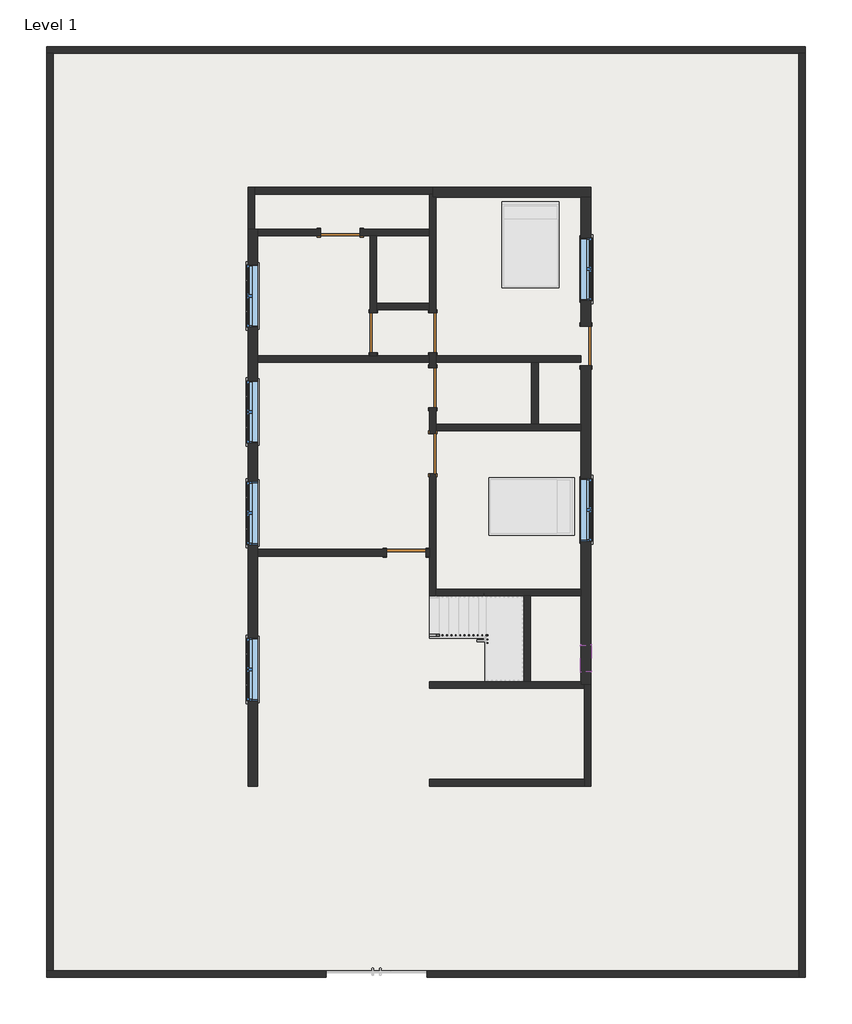
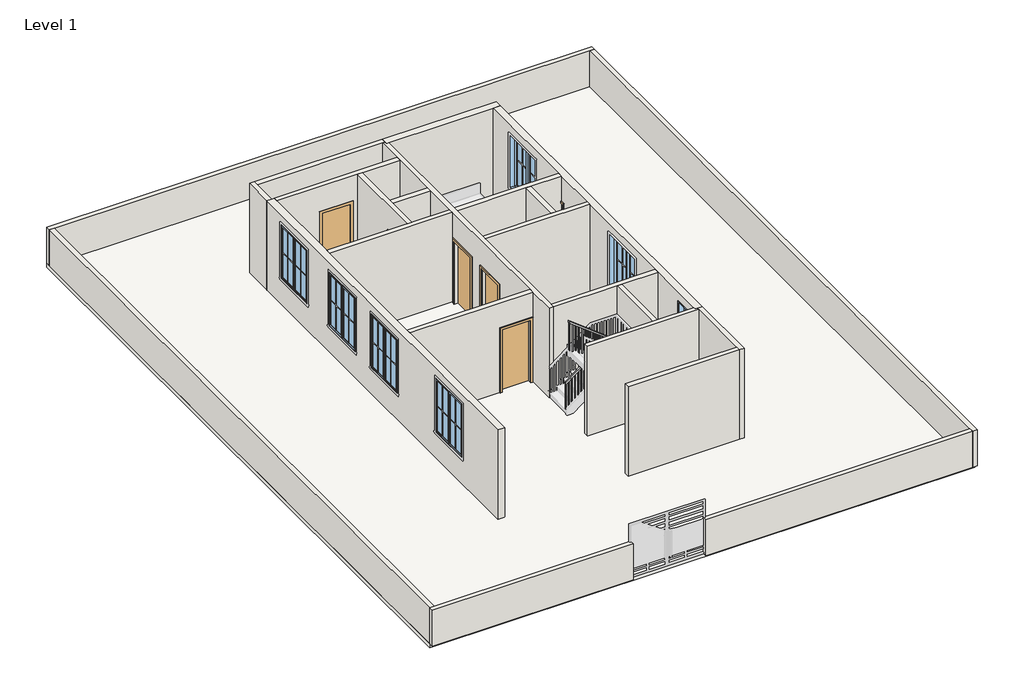
# One storey, part 1 of 2: 23 walls, 7 doors, 7 windows, 1 railing, 1 slab.
"""IFC4 building model written with IfcOpenShell, lengths in millimetres."""

from ifc_helpers import new_model, si_unit, frame, origin, origin_with_axes, place, context, project, spatial, polyline, outline, extrude, faceted_brep, transform, mapped, element, save
from components import door_686f89d2, door_16372e1c, door_0ca8825f, window_9ac97e1a, window_f2d8fef0

model = new_model("IFC4")

# Units and contexts
model_context = context("Model", 3, world=origin())
ifc_project = project(units=[si_unit("LENGTHUNIT", "METRE", prefix="MILLI")], contexts=[model_context])

# Site, building, storey
site = spatial("IfcSite", under=ifc_project)
building = spatial("IfcBuilding", under=site)
storey = spatial("IfcBuildingStorey", under=building, Name="Level 1", Elevation=0.0)

# Doors
placement = place(None, origin())
door_shape = door_686f89d2(model_context)
element("IfcDoor", 1, ObjectType="Single-Flush : 36\" x 84\"", at=placement, inside=storey, context=model_context, shape_type="MappedRepresentation", body=[
    mapped(door_shape, transform((-2318.0415352, 3143.9226491, 0.0), x_axis=(0.0, -1.0, 0.0), y_axis=(1.0, 0.0, 0.0), z_axis=(0.0, 0.0, 1.0))),
])
element("IfcDoor", 2, ObjectType="Single-Flush : 36\" x 84\"", at=placement, inside=storey, context=model_context, shape_type="MappedRepresentation", body=[
    mapped(door_shape, transform((-946.4415352, 3143.7222669, 0.0), x_axis=(0.0, 1.0, 0.0), y_axis=(-1.0, 0.0, 0.0), z_axis=(0.0, 0.0, 1.0))),
])
element("IfcDoor", 3, ObjectType="Single-Flush : 36\" x 84\"", at=placement, inside=storey, context=model_context, shape_type="MappedRepresentation", body=[
    mapped(door_shape, transform((-946.4415352, 1874.1230313, 0.0), x_axis=(0.0, 1.0, 0.0), y_axis=(-1.0, 0.0, 0.0), z_axis=(0.0, 0.0, 1.0))),
])
element("IfcDoor", 4, ObjectType="Single-Flush : 36\" x 84\"", at=placement, inside=storey, context=model_context, shape_type="MappedRepresentation", body=[
    mapped(door_shape, transform((-946.4415352, 350.1230313, 0.0), x_axis=(0.0, 1.0, 0.0), y_axis=(-1.0, 0.0, 0.0), z_axis=(0.0, 0.0, 1.0))),
])
element("IfcDoor", 5, ObjectType="Single-Flush : 36\" x 84\"", at=placement, inside=storey, context=model_context, shape_type="MappedRepresentation", body=[
    mapped(door_shape, transform((-3080.0415352, 5453.9645078, 0.0), x_axis=(1.0, 0.0, 0.0), y_axis=(0.0, 1.0, 0.0), z_axis=(0.0, 0.0, 1.0))),
])
door_2_shape = door_16372e1c(model_context)
element("IfcDoor", 6, ObjectType="Single-Flush : 36\" x 84\"", at=placement, inside=storey, context=model_context, shape_type="MappedRepresentation", body=[
    mapped(door_2_shape, transform((-1556.0415352, -1935.8769687, 0.0), x_axis=(1.0, 0.0, 0.0), y_axis=(0.0, 1.0, 0.0), z_axis=(0.0, 0.0, 1.0))),
])
door_3_shape = door_0ca8825f(model_context)
element("IfcDoor", 7, ObjectType="Single-Flush : 36\" x 84\"", at=placement, inside=storey, context=model_context, shape_type="MappedRepresentation", body=[
    mapped(door_3_shape, transform((2596.8584648, 2839.3230313, 0.0), x_axis=(0.0, -1.0, 0.0), y_axis=(1.0, 0.0, 0.0), z_axis=(0.0, 0.0, 1.0))),
])

# Railing
element("IfcRailing", 8, ObjectType="Handrail - Rectangular", at=placement, inside=storey, context=model_context, shape_type="SolidModel", body=[
    faceted_brep([(-1022.6415352, -3810.4539367, 1083.7333333), (-1022.6415352, -3810.4539367, 1019.5783974), (-1022.6415352, -3861.2539367, 1019.5783974), (-1022.6415352, -3861.2539367, 1083.7333333), (218.4221038, -3810.4539367, 2040.9605883), (269.2221038, -3810.4539367, 2015.9874824), (269.2221038, -3861.2539367, 2015.9874824), (218.4221038, -3861.2539367, 2040.9605883), (218.4221038, -3810.4539367, 2099.7333333), (269.2221038, -3810.4539367, 2048.9333333), (269.2221038, -3861.2539367, 2048.9333333), (218.4221038, -3861.2539367, 2099.7333333), (345.4221038, -3810.4539367, 2099.7333333), (345.4221038, -3810.4539367, 2048.9333333), (294.6221038, -3861.2539367, 2048.9333333), (294.6221038, -3861.2539367, 2099.7333333), (345.4221038, -3937.4539367, 2099.7333333), (345.4221038, -3937.4539367, 2048.9333333), (294.6221038, -3937.4539367, 2048.9333333), (294.6221038, -3937.4539367, 2099.7333333), (345.4221038, -3993.2769687, 2099.7333333), (294.6221038, -3993.2769687, 2099.7333333), (294.6221038, -4044.0769687, 2048.9333333), (345.4221038, -4044.0769687, 2048.9333333)], [[[0, 1, 2, 3]], [[1, 0, 4, 5]], [[2, 1, 5, 6]], [[3, 2, 6, 7]], [[0, 3, 7, 4]], [[5, 4, 8, 9]], [[6, 5, 9, 10]], [[7, 6, 10, 11]], [[4, 7, 11, 8]], [[9, 8, 12, 13]], [[10, 9, 13, 14]], [[11, 10, 14, 15]], [[8, 11, 15, 12]], [[13, 12, 16, 17]], [[14, 13, 17, 18]], [[15, 14, 18, 19]], [[12, 15, 19, 16]], [[20, 21, 22, 23]], [[17, 16, 20, 23]], [[18, 17, 23, 22]], [[19, 18, 22, 21]], [[16, 19, 21, 20]]]),
    faceted_brep([(345.4221038, -3993.2769687, 2099.7333333), (345.4221038, -4044.0769687, 2048.9333333), (294.6221038, -4044.0769687, 2048.9333333), (294.6221038, -3993.2769687, 2099.7333333), (345.4221038, -3993.2769687, 2229.8848366), (294.6221038, -3993.2769687, 2204.9117307), (294.6221038, -4044.0769687, 2204.9117307), (345.4221038, -4044.0769687, 2229.8848366)], [[[0, 1, 2, 3]], [[4, 5, 6, 7]], [[1, 0, 4, 7]], [[2, 1, 7, 6]], [[3, 2, 6, 5]], [[0, 3, 5, 4]]]),
    faceted_brep([(345.4221038, -4044.0769687, 2229.8848366), (294.6221038, -4044.0769687, 2204.9117307), (294.6221038, -3993.2769687, 2204.9117307), (345.4221038, -3993.2769687, 2229.8848366), (-1022.6415352, -4044.0769687, 3285.0666667), (-1022.6415352, -3993.2769687, 3285.0666667), (-1022.6415352, -3993.2769687, 3220.9117307), (-1022.6415352, -4044.0769687, 3220.9117307)], [[[0, 1, 2, 3]], [[4, 5, 6, 7]], [[1, 0, 4, 7]], [[2, 1, 7, 6]], [[3, 2, 6, 5]], [[0, 3, 5, 4]]]),
    extrude(outline(polyline([(3196.7018032, -991.2528962), (3211.3949894, -1010.3028962), (2201.3333333, -1010.3028962), (2201.3333333, -991.2528962), (3196.7018032, -991.2528962)])), frame((0.0, -4028.2019687, 0.0), z_axis=(0.0, 1.0, 0.0), x_axis=(0.0, 0.0, 1.0)), (0.0, 0.0, 1.0), 19.05),
    extrude(outline(polyline([(3118.3381431, -889.6528962), (3133.0313294, -908.7028962), (2201.3333333, -908.7028962), (2201.3333333, -889.6528962), (3118.3381431, -889.6528962)])), frame((0.0, -4028.2019687, 0.0), z_axis=(0.0, 1.0, 0.0), x_axis=(0.0, 0.0, 1.0)), (0.0, 0.0, 1.0), 19.05),
    extrude(outline(polyline([(3039.9744831, -788.0528962), (3054.6676694, -807.1028962), (2201.3333333, -807.1028962), (2201.3333333, -788.0528962), (3039.9744831, -788.0528962)])), frame((0.0, -4028.2019687, 0.0), z_axis=(0.0, 1.0, 0.0), x_axis=(0.0, 0.0, 1.0)), (0.0, 0.0, 1.0), 19.05),
    extrude(outline(polyline([(2961.6108231, -686.4528962), (2976.3040093, -705.5028962), (2032.0, -705.5028962), (2032.0, -686.4528962), (2961.6108231, -686.4528962)])), frame((0.0, -4028.2019687, 0.0), z_axis=(0.0, 1.0, 0.0), x_axis=(0.0, 0.0, 1.0)), (0.0, 0.0, 1.0), 19.05),
    extrude(outline(polyline([(2883.247163, -584.8528962), (2897.9403493, -603.9028962), (2032.0, -603.9028962), (2032.0, -584.8528962), (2883.247163, -584.8528962)])), frame((0.0, -4028.2019687, 0.0), z_axis=(0.0, 1.0, 0.0), x_axis=(0.0, 0.0, 1.0)), (0.0, 0.0, 1.0), 19.05),
    extrude(outline(polyline([(2804.883503, -483.2528962), (2819.5766892, -502.3028962), (1862.6666667, -502.3028962), (1862.6666667, -483.2528962), (2804.883503, -483.2528962)])), frame((0.0, -4028.2019687, 0.0), z_axis=(0.0, 1.0, 0.0), x_axis=(0.0, 0.0, 1.0)), (0.0, 0.0, 1.0), 19.05),
    extrude(outline(polyline([(2726.5198429, -381.6528962), (2741.2130292, -400.7028962), (1862.6666667, -400.7028962), (1862.6666667, -381.6528962), (2726.5198429, -381.6528962)])), frame((0.0, -4028.2019687, 0.0), z_axis=(0.0, 1.0, 0.0), x_axis=(0.0, 0.0, 1.0)), (0.0, 0.0, 1.0), 19.05),
    extrude(outline(polyline([(2648.1561829, -280.0528962), (2662.8493691, -299.1028962), (1693.3333333, -299.1028962), (1693.3333333, -280.0528962), (2648.1561829, -280.0528962)])), frame((0.0, -4028.2019687, 0.0), z_axis=(0.0, 1.0, 0.0), x_axis=(0.0, 0.0, 1.0)), (0.0, 0.0, 1.0), 19.05),
    extrude(outline(polyline([(2569.7925228, -178.4528962), (2584.4857091, -197.5028962), (1693.3333333, -197.5028962), (1693.3333333, -178.4528962), (2569.7925228, -178.4528962)])), frame((0.0, -4028.2019687, 0.0), z_axis=(0.0, 1.0, 0.0), x_axis=(0.0, 0.0, 1.0)), (0.0, 0.0, 1.0), 19.05),
    extrude(outline(polyline([(2491.4288628, -76.8528962), (2506.122049, -95.9028962), (1524.0, -95.9028962), (1524.0, -76.8528962), (2491.4288628, -76.8528962)])), frame((0.0, -4028.2019687, 0.0), z_axis=(0.0, 1.0, 0.0), x_axis=(0.0, 0.0, 1.0)), (0.0, 0.0, 1.0), 19.05),
    extrude(outline(polyline([(2413.0652027, 24.7471038), (2427.758389, 5.6971038), (1524.0, 5.6971038), (1524.0, 24.7471038), (2413.0652027, 24.7471038)])), frame((0.0, -4028.2019687, 0.0), z_axis=(0.0, 1.0, 0.0), x_axis=(0.0, 0.0, 1.0)), (0.0, 0.0, 1.0), 19.05),
    extrude(outline(polyline([(2334.7015427, 126.3471038), (2349.3947289, 107.2971038), (1524.0, 107.2971038), (1524.0, 126.3471038), (2334.7015427, 126.3471038)])), frame((0.0, -4028.2019687, 0.0), z_axis=(0.0, 1.0, 0.0), x_axis=(0.0, 0.0, 1.0)), (0.0, 0.0, 1.0), 19.05),
    extrude(outline(polyline([(2256.3378826, 227.9471038), (2271.0310689, 208.8971038), (1354.6666667, 208.8971038), (1354.6666667, 227.9471038), (2256.3378826, 227.9471038)])), frame((0.0, -4028.2019687, 0.0), z_axis=(0.0, 1.0, 0.0), x_axis=(0.0, 0.0, 1.0)), (0.0, 0.0, 1.0), 19.05),
    extrude(outline(polyline([(310.4971038, -3927.9289367), (329.5471038, -3927.9289367), (329.5471038, -3946.9789367), (310.4971038, -3946.9789367), (310.4971038, -3927.9289367)])), frame((0.0, 0.0, 1185.3333333), z_axis=(0.0, 0.0, 1.0), x_axis=(1.0, 0.0, 0.0)), (0.0, 0.0, 1.0), 863.6),
    extrude(outline(polyline([(288.6334648, -3845.3789367), (288.6334648, -3826.3289367), (307.6834648, -3826.3289367), (307.6834648, -3845.3789367), (288.6334648, -3845.3789367)])), frame((0.0, 0.0, 1185.3333333), z_axis=(0.0, 0.0, 1.0), x_axis=(1.0, 0.0, 0.0)), (0.0, 0.0, 1.0), 863.6),
    extrude(outline(polyline([(1967.2889111, 206.0834648), (1952.5957248, 187.0334648), (1016.0, 187.0334648), (1016.0, 206.0834648), (1967.2889111, 206.0834648)])), frame((0.0, -3845.3789367, 0.0), z_axis=(0.0, 1.0, 0.0), x_axis=(0.0, 0.0, 1.0)), (0.0, 0.0, 1.0), 19.05),
    extrude(outline(polyline([(1888.925251, 104.4834648), (1874.2320648, 85.4334648), (846.6666667, 85.4334648), (846.6666667, 104.4834648), (1888.925251, 104.4834648)])), frame((0.0, -3845.3789367, 0.0), z_axis=(0.0, 1.0, 0.0), x_axis=(0.0, 0.0, 1.0)), (0.0, 0.0, 1.0), 19.05),
    extrude(outline(polyline([(1810.561591, 2.8834648), (1795.8684047, -16.1665352), (846.6666667, -16.1665352), (846.6666667, 2.8834648), (1810.561591, 2.8834648)])), frame((0.0, -3845.3789367, 0.0), z_axis=(0.0, 1.0, 0.0), x_axis=(0.0, 0.0, 1.0)), (0.0, 0.0, 1.0), 19.05),
    extrude(outline(polyline([(1732.1979309, -98.7165352), (1717.5047447, -117.7665352), (846.6666667, -117.7665352), (846.6666667, -98.7165352), (1732.1979309, -98.7165352)])), frame((0.0, -3845.3789367, 0.0), z_axis=(0.0, 1.0, 0.0), x_axis=(0.0, 0.0, 1.0)), (0.0, 0.0, 1.0), 19.05),
    extrude(outline(polyline([(1653.8342709, -200.3165352), (1639.1410846, -219.3665352), (677.3333333, -219.3665352), (677.3333333, -200.3165352), (1653.8342709, -200.3165352)])), frame((0.0, -3845.3789367, 0.0), z_axis=(0.0, 1.0, 0.0), x_axis=(0.0, 0.0, 1.0)), (0.0, 0.0, 1.0), 19.05),
    extrude(outline(polyline([(1575.4706109, -301.9165352), (1560.7774246, -320.9665352), (677.3333333, -320.9665352), (677.3333333, -301.9165352), (1575.4706109, -301.9165352)])), frame((0.0, -3845.3789367, 0.0), z_axis=(0.0, 1.0, 0.0), x_axis=(0.0, 0.0, 1.0)), (0.0, 0.0, 1.0), 19.05),
    extrude(outline(polyline([(1497.1069508, -403.5165352), (1482.4137645, -422.5665352), (508.0, -422.5665352), (508.0, -403.5165352), (1497.1069508, -403.5165352)])), frame((0.0, -3845.3789367, 0.0), z_axis=(0.0, 1.0, 0.0), x_axis=(0.0, 0.0, 1.0)), (0.0, 0.0, 1.0), 19.05),
    extrude(outline(polyline([(1418.7432908, -505.1165352), (1404.0501045, -524.1665352), (508.0, -524.1665352), (508.0, -505.1165352), (1418.7432908, -505.1165352)])), frame((0.0, -3845.3789367, 0.0), z_axis=(0.0, 1.0, 0.0), x_axis=(0.0, 0.0, 1.0)), (0.0, 0.0, 1.0), 19.05),
    extrude(outline(polyline([(1340.3796307, -606.7165352), (1325.6864445, -625.7665352), (338.6666667, -625.7665352), (338.6666667, -606.7165352), (1340.3796307, -606.7165352)])), frame((0.0, -3845.3789367, 0.0), z_axis=(0.0, 1.0, 0.0), x_axis=(0.0, 0.0, 1.0)), (0.0, 0.0, 1.0), 19.05),
    extrude(outline(polyline([(1262.0159707, -708.3165352), (1247.3227844, -727.3665352), (338.6666667, -727.3665352), (338.6666667, -708.3165352), (1262.0159707, -708.3165352)])), frame((0.0, -3845.3789367, 0.0), z_axis=(0.0, 1.0, 0.0), x_axis=(0.0, 0.0, 1.0)), (0.0, 0.0, 1.0), 19.05),
    extrude(outline(polyline([(1183.6523106, -809.9165352), (1168.9591244, -828.9665352), (169.3333333, -828.9665352), (169.3333333, -809.9165352), (1183.6523106, -809.9165352)])), frame((0.0, -3845.3789367, 0.0), z_axis=(0.0, 1.0, 0.0), x_axis=(0.0, 0.0, 1.0)), (0.0, 0.0, 1.0), 19.05),
    extrude(outline(polyline([(1105.2886506, -911.5165352), (1090.5954643, -930.5665352), (169.3333333, -930.5665352), (169.3333333, -911.5165352), (1105.2886506, -911.5165352)])), frame((0.0, -3845.3789367, 0.0), z_axis=(0.0, 1.0, 0.0), x_axis=(0.0, 0.0, 1.0)), (0.0, 0.0, 1.0), 19.05),
    extrude(outline(polyline([(310.4971038, -4009.1519687), (329.5471038, -4009.1519687), (329.5471038, -4028.2019687), (310.4971038, -4028.2019687), (310.4971038, -4009.1519687)])), frame((0.0, 0.0, 1185.3333333), z_axis=(0.0, 0.0, 1.0), x_axis=(1.0, 0.0, 0.0)), (0.0, 0.0, 1.0), 863.6),
    extrude(outline(polyline([(310.4971038, -3845.3789367), (310.4971038, -3826.3289367), (329.5471038, -3826.3289367), (329.5471038, -3845.3789367), (310.4971038, -3845.3789367)])), frame((0.0, 0.0, 1185.3333333), z_axis=(0.0, 0.0, 1.0), x_axis=(1.0, 0.0, 0.0)), (0.0, 0.0, 1.0), 863.6),
    extrude(outline(polyline([(3206.2185445, -1003.5915352), (3220.9117307, -1022.6415352), (2201.3333333, -1022.6415352), (2201.3333333, -1003.5915352), (3206.2185445, -1003.5915352)])), frame((0.0, -4028.2019687, 0.0), z_axis=(0.0, 1.0, 0.0), x_axis=(0.0, 0.0, 1.0)), (0.0, 0.0, 1.0), 19.05),
    extrude(outline(polyline([(1034.2715837, -1003.5915352), (1019.5783974, -1022.6415352), (169.3333333, -1022.6415352), (169.3333333, -1003.5915352), (1034.2715837, -1003.5915352)])), frame((0.0, -3845.3789367, 0.0), z_axis=(0.0, 1.0, 0.0), x_axis=(0.0, 0.0, 1.0)), (0.0, 0.0, 1.0), 19.05),
])

# Slab
element("IfcSlab", 9, ObjectType="FLOOR 6\"", at=placement, inside=storey, context=model_context, shape_type="SweptSolid", body=[
    extrude(outline(polyline([(7660.9863196, 9750.111972), (7660.9863196, -11585.888028), (-9865.0136804, -11585.888028), (-9865.0136804, 9750.111972), (7660.9863196, 9750.111972)])), frame((0.0, 0.0, -152.4), z_axis=(0.0, 0.0, 1.0), x_axis=(1.0, 0.0, 0.0)), (0.0, 0.0, 1.0), 152.4),
])

# Walls
element("IfcWall", 10, ObjectType="WALL 6\"", at=placement, inside=storey, context=model_context, shape_type="Brep", body=[
    faceted_brep([(-5061.2415352, 5531.7230313, 0.0), (-5061.2415352, 6344.5230313, 0.0), (-5061.2415352, 6496.9230313, 0.0), (-5061.2415352, 6496.9230313, 3048.0), (-5061.2415352, 6344.5230313, 3048.0), (-5061.2415352, 5531.7230313, 3048.0), (-5213.6415352, 5531.7230313, 0.0), (-5213.6415352, 5531.7230313, 3048.0), (-5213.6415352, 6496.9230313, 3048.0), (-5213.6415352, 6496.9230313, 0.0)], [[[0, 1, 2, 3, 4, 5]], [[6, 7, 8, 9]], [[2, 1, 0, 6, 9]], [[0, 5, 7, 6]], [[3, 2, 9, 8]], [[5, 4, 3, 8, 7]]]),
])
element("IfcWall", 11, ObjectType="WALL 6\"", at=placement, inside=storey, context=model_context, shape_type="Brep", body=[
    faceted_brep([(-5061.2415352, 6344.5230313, 0.0), (-1022.6415352, 6344.5230313, 0.0), (-946.4415352, 6344.5230313, 0.0), (-946.4415352, 6344.5230313, 3048.0), (-1022.6415352, 6344.5230313, 3048.0), (-5061.2415352, 6344.5230313, 3048.0), (-5061.2415352, 6496.9230313, 0.0), (-5061.2415352, 6496.9230313, 3048.0), (-946.4415352, 6496.9230313, 3048.0), (-946.4415352, 6496.9230313, 0.0)], [[[0, 1, 2, 3, 4, 5]], [[6, 7, 8, 9]], [[2, 1, 0, 6, 9]], [[3, 2, 9, 8]], [[0, 5, 7, 6]], [[5, 4, 3, 8, 7]]]),
])
element("IfcWall", 12, ObjectType="WALL 6\"", at=placement, inside=storey, context=model_context, shape_type="Brep", body=[
    faceted_brep([(-1022.6415352, 1416.9230313, 0.0), (-1022.6415352, 807.3230313, 0.0), (-1022.6415352, 807.3230313, 2133.6), (-1022.6415352, -107.0769687, 2133.6), (-1022.6415352, -107.0769687, 0.0), (-1022.6415352, -1859.6769687, 0.0), (-1022.6415352, -2012.0769687, 0.0), (-1022.6415352, -2926.4769687, 0.0), (-1022.6415352, -2926.4769687, 3048.0), (-1022.6415352, -2012.0769687, 3048.0), (-1022.6415352, -1859.6769687, 3048.0), (-1022.6415352, 2458.3230313, 3048.0), (-1022.6415352, 2610.7230313, 3048.0), (-1022.6415352, 3677.1222669, 3048.0), (-1022.6415352, 3829.5222669, 3048.0), (-1022.6415352, 5377.7645078, 3048.0), (-1022.6415352, 5530.1645078, 3048.0), (-1022.6415352, 6344.5230313, 3048.0), (-1022.6415352, 6344.5230313, 0.0), (-1022.6415352, 5530.1645078, 0.0), (-1022.6415352, 5377.7645078, 0.0), (-1022.6415352, 3829.5222669, 0.0), (-1022.6415352, 3677.1222669, 0.0), (-1022.6415352, 3600.9222669, 0.0), (-1022.6415352, 3600.9222669, 2133.6), (-1022.6415352, 2686.5222669, 2133.6), (-1022.6415352, 2686.5222669, 0.0), (-1022.6415352, 2610.7230313, 0.0), (-1022.6415352, 2458.3230313, 0.0), (-1022.6415352, 2331.3230313, 0.0), (-1022.6415352, 2331.3230313, 2133.6), (-1022.6415352, 1416.9230313, 2133.6), (-870.2415352, 807.3230313, 2133.6), (-870.2415352, 807.3230313, 0.0), (-870.2415352, 883.5230313, 0.0), (-870.2415352, 1035.9230313, 0.0), (-870.2415352, 1416.9230313, 0.0), (-870.2415352, 1416.9230313, 2133.6), (-870.2415352, 2331.3230313, 2133.6), (-870.2415352, 2331.3230313, 0.0), (-870.2415352, 2458.3230313, 0.0), (-870.2415352, 2610.7230313, 0.0), (-870.2415352, 2686.5222669, 0.0), (-870.2415352, 2686.5222669, 2133.6), (-870.2415352, 3600.9222669, 2133.6), (-870.2415352, 3600.9222669, 0.0), (-870.2415352, 6268.3230313, 0.0), (-870.2415352, 6268.3230313, 3048.0), (-870.2415352, 2610.7230313, 3048.0), (-870.2415352, 2458.3230313, 3048.0), (-870.2415352, 1035.9230313, 3048.0), (-870.2415352, 883.5230313, 3048.0), (-870.2415352, -2774.0769687, 3048.0), (-870.2415352, -2926.4769687, 3048.0), (-870.2415352, -2926.4769687, 0.0), (-870.2415352, -2774.0769687, 0.0), (-870.2415352, -107.0769687, 0.0), (-870.2415352, -107.0769687, 2133.6), (-946.4415352, 6344.5230313, 0.0), (-946.4415352, 6268.3230313, 0.0), (-946.4415352, 6344.5230313, 3048.0), (-946.4415352, 6268.3230313, 3048.0)], [[[0, 1, 2, 3, 4, 5, 6, 7, 8, 9, 10, 11, 12, 13, 14, 15, 16, 17, 18, 19, 20, 21, 22, 23, 24, 25, 26, 27, 28, 29, 30, 31]], [[32, 33, 34, 35, 36, 37, 38, 39, 40, 41, 42, 43, 44, 45, 46, 47, 48, 49, 50, 51, 52, 53, 54, 55, 56, 57]], [[46, 45, 23, 22, 21, 20, 19, 18, 58, 59]], [[42, 41, 40, 39, 29, 28, 27, 26]], [[56, 55, 54, 7, 6, 5, 4]], [[36, 35, 34, 33, 1, 0]], [[18, 17, 60, 58]], [[60, 61, 59, 58]], [[61, 47, 46, 59]], [[8, 7, 54, 53]], [[24, 23, 45, 44]], [[25, 24, 44, 43]], [[26, 25, 43, 42]], [[30, 29, 39, 38]], [[31, 30, 38, 37]], [[0, 31, 37, 36]], [[2, 1, 33, 32]], [[3, 2, 32, 57]], [[4, 3, 57, 56]], [[17, 16, 15, 14, 13, 12, 11, 10, 9, 8, 53, 52, 51, 50, 49, 48, 47, 61, 60]]]),
])
element("IfcWall", 13, ObjectType="WALL 6\"", at=placement, inside=storey, context=model_context, shape_type="Brep", body=[
    faceted_brep([(2482.5584648, -2774.0769687, 0.0), (-870.2415352, -2774.0769687, 0.0), (-870.2415352, -2774.0769687, 3048.0), (2482.5584648, -2774.0769687, 3048.0), (2482.5584648, -2926.4769687, 0.0), (2482.5584648, -2926.4769687, 3048.0), (1314.1584648, -2926.4769687, 3048.0), (1161.7584648, -2926.4769687, 3048.0), (-870.2415352, -2926.4769687, 3048.0), (-870.2415352, -2926.4769687, 0.0), (1161.7584648, -2926.4769687, 0.0), (1314.1584648, -2926.4769687, 0.0)], [[[0, 1, 2, 3]], [[4, 5, 6, 7, 8, 9, 10, 11]], [[1, 0, 4, 11, 10, 9]], [[2, 1, 9, 8]], [[0, 3, 5, 4]], [[3, 2, 8, 7, 6, 5]]]),
])
element("IfcWall", 14, ObjectType="WALL 6\"", at=placement, inside=storey, context=model_context, shape_type="Brep", body=[
    faceted_brep([(2558.7584648, -4983.8769687, 0.0), (2558.7584648, -5060.0769687, 0.0), (2558.7584648, -7168.2769687, 0.0), (2558.7584648, -7320.6769687, 0.0), (2558.7584648, -7320.6769687, 3048.0), (2558.7584648, -7168.2769687, 3048.0), (2558.7584648, -5060.0769687, 3048.0), (2558.7584648, -4983.8769687, 3048.0), (2711.1584648, -4983.8769687, 0.0), (2711.1584648, -4983.8769687, 3048.0), (2711.1584648, -7320.6769687, 3048.0), (2711.1584648, -7320.6769687, 0.0)], [[[0, 1, 2, 3, 4, 5, 6, 7]], [[8, 9, 10, 11]], [[3, 2, 1, 0, 8, 11]], [[0, 7, 9, 8]], [[4, 3, 11, 10]], [[7, 6, 5, 4, 10, 9]]]),
])
element("IfcWall", 15, ObjectType="WALL 6\"", at=placement, inside=storey, context=model_context, shape_type="SweptSolid", body=[
    extrude(outline(polyline([(-1022.6415352, -7168.2769687), (2558.7584648, -7168.2769687), (2558.7584648, -7320.6769687), (-1022.6415352, -7320.6769687), (-1022.6415352, -7168.2769687)])), origin_with_axes(), (0.0, 0.0, 1.0), 3048.0),
])
element("IfcWall", 16, ObjectType="WALL 6\"", at=placement, inside=storey, context=model_context, shape_type="Brep", body=[
    faceted_brep([(2482.5584648, -4907.6769687, 0.0), (1314.1584648, -4907.6769687, 0.0), (1161.7584648, -4907.6769687, 0.0), (-1022.6415352, -4907.6769687, 0.0), (-1022.6415352, -4907.6769687, 3048.0), (1161.7584648, -4907.6769687, 3048.0), (1314.1584648, -4907.6769687, 3048.0), (2482.5584648, -4907.6769687, 3048.0), (2558.7584648, -5060.0769687, 0.0), (2558.7584648, -5060.0769687, 3048.0), (-1022.6415352, -5060.0769687, 3048.0), (-1022.6415352, -5060.0769687, 0.0), (2482.5584648, -4983.8769687, 0.0), (2558.7584648, -4983.8769687, 0.0), (2482.5584648, -4983.8769687, 3048.0), (2558.7584648, -4983.8769687, 3048.0)], [[[0, 1, 2, 3, 4, 5, 6, 7]], [[8, 9, 10, 11]], [[3, 2, 1, 0, 12, 13, 8, 11]], [[4, 3, 11, 10]], [[0, 7, 14, 12]], [[14, 15, 13, 12]], [[15, 9, 8, 13]], [[7, 6, 5, 4, 10, 9, 15, 14]]]),
])
element("IfcWall", 17, ObjectType="WALL 6\"", at=placement, inside=storey, context=model_context, shape_type="SweptSolid", body=[
    extrude(outline(polyline([(1161.7584648, -4907.6769687), (1161.7584648, -2926.4769687), (1314.1584648, -2926.4769687), (1314.1584648, -4907.6769687), (1161.7584648, -4907.6769687)])), origin_with_axes(), (0.0, 0.0, 1.0), 3048.0),
])
element("IfcWall", 18, ObjectType="WALL 6\"", at=placement, inside=storey, context=model_context, shape_type="SweptSolid", body=[
    extrude(outline(polyline([(2133.6, -1098.8415352), (0.0, -1098.8415352), (0.0, -1022.6415352), (3048.0, -1022.6415352), (3048.0, -4985.0415352), (0.0, -4985.0415352), (0.0, -2013.2415352), (2133.6, -2013.2415352), (2133.6, -1098.8415352)])), frame((0.0, -2012.0769687, 0.0), z_axis=(0.0, 1.0, 0.0), x_axis=(0.0, 0.0, 1.0)), (0.0, 0.0, 1.0), 152.4),
])
element("IfcWall", 19, ObjectType="WALL 6\"", at=placement, inside=storey, context=model_context, shape_type="Brep", body=[
    faceted_brep([(2482.5584648, 2458.3230313, 0.0), (2482.5584648, 2458.3230313, 3048.0), (1491.9584648, 2458.3230313, 3048.0), (1339.5584648, 2458.3230313, 3048.0), (-870.2415352, 2458.3230313, 3048.0), (-870.2415352, 2458.3230313, 0.0), (1339.5584648, 2458.3230313, 0.0), (1491.9584648, 2458.3230313, 0.0), (2482.5584648, 2610.7230313, 3048.0), (2482.5584648, 2610.7230313, 0.0), (-870.2415352, 2610.7230313, 0.0), (-870.2415352, 2610.7230313, 3048.0)], [[[0, 1, 2, 3, 4, 5, 6, 7]], [[8, 9, 10, 11]], [[9, 0, 7, 6, 5, 10]], [[1, 0, 9, 8]], [[5, 4, 11, 10]], [[1, 8, 11, 4, 3, 2]]]),
    faceted_brep([(-4985.0415352, 2458.3230313, 3048.0), (-4985.0415352, 2458.3230313, 0.0), (-1022.6415352, 2458.3230313, 0.0), (-1022.6415352, 2458.3230313, 3048.0), (-4985.0415352, 2610.7230313, 0.0), (-4985.0415352, 2610.7230313, 3048.0), (-2394.2415352, 2610.7230313, 3048.0), (-2241.8415352, 2610.7230313, 3048.0), (-1022.6415352, 2610.7230313, 3048.0), (-1022.6415352, 2610.7230313, 0.0), (-2241.8415352, 2610.7230313, 0.0), (-2394.2415352, 2610.7230313, 0.0)], [[[0, 1, 2, 3]], [[4, 5, 6, 7, 8, 9, 10, 11]], [[1, 4, 11, 10, 9, 2]], [[1, 0, 5, 4]], [[3, 2, 9, 8]], [[5, 0, 3, 8, 7, 6]]]),
])
element("IfcWall", 20, ObjectType="WALL 6\"", at=placement, inside=storey, context=model_context, shape_type="Brep", body=[
    faceted_brep([(-2622.8415352, 5377.7645078, 2133.6), (-2622.8415352, 5377.7645078, 0.0), (-2394.2415352, 5377.7645078, 0.0), (-2241.8415352, 5377.7645078, 0.0), (-1022.6415352, 5377.7645078, 0.0), (-1022.6415352, 5377.7645078, 3048.0), (-2241.8415352, 5377.7645078, 3048.0), (-2394.2415352, 5377.7645078, 3048.0), (-4985.0415352, 5377.7645078, 3048.0), (-4985.0415352, 5377.7645078, 0.0), (-3537.2415352, 5377.7645078, 0.0), (-3537.2415352, 5377.7645078, 2133.6), (-1022.6415352, 5530.1645078, 0.0), (-2622.8415352, 5530.1645078, 0.0), (-2622.8415352, 5530.1645078, 2133.6), (-3537.2415352, 5530.1645078, 2133.6), (-3537.2415352, 5530.1645078, 0.0), (-4985.0415352, 5530.1645078, 0.0), (-4985.0415352, 5530.1645078, 3048.0), (-1022.6415352, 5530.1645078, 3048.0)], [[[0, 1, 2, 3, 4, 5, 6, 7, 8, 9, 10, 11]], [[12, 13, 14, 15, 16, 17, 18, 19]], [[10, 9, 17, 16]], [[4, 3, 2, 1, 13, 12]], [[9, 8, 18, 17]], [[5, 4, 12, 19]], [[14, 13, 1, 0]], [[15, 14, 0, 11]], [[16, 15, 11, 10]], [[8, 7, 6, 5, 19, 18]]]),
])
element("IfcWall", 21, ObjectType="WALL 6\"", at=placement, inside=storey, context=model_context, shape_type="Brep", body=[
    faceted_brep([(-2394.2415352, 2686.7226491, 2133.6), (-2394.2415352, 2686.7226491, 0.0), (-2394.2415352, 2610.7230313, 0.0), (-2394.2415352, 2610.7230313, 3048.0), (-2394.2415352, 5377.7645078, 3048.0), (-2394.2415352, 5377.7645078, 0.0), (-2394.2415352, 3601.1226491, 0.0), (-2394.2415352, 3601.1226491, 2133.6), (-2241.8415352, 2610.7230313, 0.0), (-2241.8415352, 2686.7226491, 0.0), (-2241.8415352, 2686.7226491, 2133.6), (-2241.8415352, 3601.1226491, 2133.6), (-2241.8415352, 3601.1226491, 0.0), (-2241.8415352, 3677.1222669, 0.0), (-2241.8415352, 3829.5222669, 0.0), (-2241.8415352, 5377.7645078, 0.0), (-2241.8415352, 5377.7645078, 3048.0), (-2241.8415352, 3829.5222669, 3048.0), (-2241.8415352, 3677.1222669, 3048.0), (-2241.8415352, 2610.7230313, 3048.0)], [[[0, 1, 2, 3, 4, 5, 6, 7]], [[8, 9, 10, 11, 12, 13, 14, 15, 16, 17, 18, 19]], [[6, 5, 15, 14, 13, 12]], [[2, 1, 9, 8]], [[3, 2, 8, 19]], [[5, 4, 16, 15]], [[10, 9, 1, 0]], [[11, 10, 0, 7]], [[12, 11, 7, 6]], [[4, 3, 19, 18, 17, 16]]]),
])
element("IfcWall", 22, ObjectType="WALL 6\"", at=placement, inside=storey, context=model_context, shape_type="SweptSolid", body=[
    extrude(outline(polyline([(-1022.6415352, 3677.1222669), (-2241.8415352, 3677.1222669), (-2241.8415352, 3829.5222669), (-1022.6415352, 3829.5222669), (-1022.6415352, 3677.1222669)])), origin_with_axes(), (0.0, 0.0, 1.0), 3048.0),
])
element("IfcWall", 23, ObjectType="WALL 6\"", at=placement, inside=storey, context=model_context, shape_type="Brep", body=[
    faceted_brep([(-870.2415352, 883.5230313, 0.0), (2482.5584648, 883.5230313, 0.0), (2482.5584648, 883.5230313, 3048.0), (-870.2415352, 883.5230313, 3048.0), (-870.2415352, 1035.9230313, 0.0), (-870.2415352, 1035.9230313, 3048.0), (1339.5584648, 1035.9230313, 3048.0), (1491.9584648, 1035.9230313, 3048.0), (2482.5584648, 1035.9230313, 3048.0), (2482.5584648, 1035.9230313, 0.0), (1491.9584648, 1035.9230313, 0.0), (1339.5584648, 1035.9230313, 0.0)], [[[0, 1, 2, 3]], [[4, 5, 6, 7, 8, 9, 10, 11]], [[1, 0, 4, 11, 10, 9]], [[2, 1, 9, 8]], [[0, 3, 5, 4]], [[3, 2, 8, 7, 6, 5]]]),
])
element("IfcWall", 24, ObjectType="WALL 6\"", at=placement, inside=storey, context=model_context, shape_type="SweptSolid", body=[
    extrude(outline(polyline([(1339.5584648, 1035.9230313), (1339.5584648, 2458.3230313), (1491.9584648, 2458.3230313), (1491.9584648, 1035.9230313), (1339.5584648, 1035.9230313)])), origin_with_axes(), (0.0, 0.0, 1.0), 3048.0),
])
element("IfcWall", 25, ObjectType="WALL 6\"", at=placement, inside=storey, context=model_context, shape_type="Brep", body=[
    faceted_brep([(-9865.0136804, 9597.711972, 0.0), (-9712.6136804, 9597.711972, 0.0), (7508.5863196, 9597.711972, 0.0), (7660.9863196, 9597.711972, 0.0), (7660.9863196, 9597.711972, 1219.2), (7508.5863196, 9597.711972, 1219.2), (-9712.6136804, 9597.711972, 1219.2), (-9865.0136804, 9597.711972, 1219.2), (-9865.0136804, 9750.111972, 0.0), (-9865.0136804, 9750.111972, 1219.2), (7660.9863196, 9750.111972, 1219.2), (7660.9863196, 9750.111972, 0.0)], [[[0, 1, 2, 3, 4, 5, 6, 7]], [[8, 9, 10, 11]], [[3, 2, 1, 0, 8, 11]], [[7, 6, 5, 4, 10, 9]], [[4, 3, 11, 10]], [[0, 7, 9, 8]]]),
])
element("IfcWall", 26, ObjectType="WALL 6\"", at=placement, inside=storey, context=model_context, shape_type="Brep", body=[
    faceted_brep([(7508.5863196, 9597.711972, 0.0), (7508.5863196, -11585.888028, 0.0), (7508.5863196, -11738.288028, 0.0), (7508.5863196, -11738.288028, 1219.2), (7508.5863196, -11585.888028, 1219.2), (7508.5863196, 9597.711972, 1219.2), (7660.9863196, 9597.711972, 0.0), (7660.9863196, 9597.711972, 1219.2), (7660.9863196, -11738.288028, 1219.2), (7660.9863196, -11738.288028, 0.0)], [[[0, 1, 2, 3, 4, 5]], [[6, 7, 8, 9]], [[2, 1, 0, 6, 9]], [[5, 4, 3, 8, 7]], [[0, 5, 7, 6]], [[3, 2, 9, 8]]]),
])
element("IfcWall", 27, ObjectType="WALL 6\"", at=placement, inside=storey, context=model_context, shape_type="SweptSolid", body=[
    extrude(outline(polyline([(-1073.4415352, -11585.888028), (7508.5863196, -11585.888028), (7508.5863196, -11738.288028), (-1073.4415352, -11738.288028), (-1073.4415352, -11585.888028)])), origin_with_axes(), (0.0, 0.0, 1.0), 1219.2),
])
element("IfcWall", 28, ObjectType="WALL 6\"", at=placement, inside=storey, context=model_context, shape_type="SweptSolid", body=[
    extrude(outline(polyline([(-9712.6136804, 9597.711972), (-9712.6136804, -11585.888028), (-9865.0136804, -11585.888028), (-9865.0136804, 9597.711972), (-9712.6136804, 9597.711972)])), origin_with_axes(), (0.0, 0.0, 1.0), 1219.2),
])
element("IfcWall", 29, ObjectType="WALL 6\"", at=placement, inside=storey, context=model_context, shape_type="Brep", body=[
    faceted_brep([(-3410.2415352, -11585.888028, 0.0), (-9712.6136804, -11585.888028, 0.0), (-9865.0136804, -11585.888028, 0.0), (-9865.0136804, -11585.888028, 1219.2), (-9712.6136804, -11585.888028, 1219.2), (-3410.2415352, -11585.888028, 1219.2), (-3410.2415352, -11738.288028, 0.0), (-3410.2415352, -11738.288028, 1219.2), (-9865.0136804, -11738.288028, 1219.2), (-9865.0136804, -11738.288028, 0.0)], [[[0, 1, 2, 3, 4, 5]], [[6, 7, 8, 9]], [[2, 1, 0, 6, 9]], [[5, 4, 3, 8, 7]], [[0, 5, 7, 6]], [[3, 2, 9, 8]]]),
])
element("IfcWall", 30, ObjectType="WALL 9\"", at=placement, inside=storey, context=model_context, shape_type="Brep", body=[
    faceted_brep([(-946.4415352, 6268.3230313, 0.0), (-870.2415352, 6268.3230313, 0.0), (2482.5584648, 6268.3230313, 0.0), (2711.1584648, 6268.3230313, 0.0), (2711.1584648, 6268.3230313, 3048.0), (2482.5584648, 6268.3230313, 3048.0), (-870.2415352, 6268.3230313, 3048.0), (-946.4415352, 6268.3230313, 3048.0), (-946.4415352, 6496.9230313, 0.0), (-946.4415352, 6496.9230313, 3048.0), (2711.1584648, 6496.9230313, 3048.0), (2711.1584648, 6496.9230313, 0.0), (-946.4415352, 6344.5230313, 0.0), (-946.4415352, 6344.5230313, 3048.0)], [[[0, 1, 2, 3, 4, 5, 6, 7]], [[8, 9, 10, 11]], [[3, 2, 1, 0, 12, 8, 11]], [[0, 7, 13, 9, 8, 12]], [[4, 3, 11, 10]], [[7, 6, 5, 4, 10, 9, 13]]]),
])
element("IfcWall", 31, ObjectType="WALL 9\"", at=placement, inside=storey, context=model_context, shape_type="Brep", body=[
    faceted_brep([(2482.5584648, 2382.1230313, 2133.6), (2482.5584648, 2382.1230313, 0.0), (2482.5584648, 1035.9230313, 0.0), (2482.5584648, 883.5230313, 0.0), (2482.5584648, -2774.0769687, 0.0), (2482.5584648, -2926.4769687, 0.0), (2482.5584648, -4907.6769687, 0.0), (2482.5584648, -4983.8769687, 0.0), (2482.5584648, -4983.8769687, 3048.0), (2482.5584648, -4907.6769687, 3048.0), (2482.5584648, -2926.4769687, 3048.0), (2482.5584648, -2774.0769687, 3048.0), (2482.5584648, 883.5230313, 3048.0), (2482.5584648, 1035.9230313, 3048.0), (2482.5584648, 2458.3230313, 3048.0), (2482.5584648, 2610.7230313, 3048.0), (2482.5584648, 6268.3230313, 3048.0), (2482.5584648, 6268.3230313, 0.0), (2482.5584648, 3296.5230313, 0.0), (2482.5584648, 3296.5230313, 2133.6), (2482.5584648, 3887.0730313, 2743.2), (2482.5584648, 3887.0730313, 914.4), (2482.5584648, 5334.8730313, 914.4), (2482.5584648, 5334.8730313, 2743.2), (2482.5584648, -1669.1769687, 2743.2), (2482.5584648, -1669.1769687, 914.4), (2482.5584648, -221.3769687, 914.4), (2482.5584648, -221.3769687, 2743.2), (2482.5584648, -4069.4769687, 2743.2), (2482.5584648, -4679.0769687, 2743.2), (2482.5584648, -4679.0769687, 2133.6), (2482.5584648, -4069.4769687, 2133.6), (2711.1584648, -4983.8769687, 0.0), (2711.1584648, 2382.1230313, 0.0), (2711.1584648, 2382.1230313, 2133.6), (2711.1584648, 3296.5230313, 2133.6), (2711.1584648, 3296.5230313, 0.0), (2711.1584648, 6268.3230313, 0.0), (2711.1584648, 6268.3230313, 3048.0), (2711.1584648, -4983.8769687, 3048.0), (2711.1584648, 3887.0730313, 2743.2), (2711.1584648, 5334.8730313, 2743.2), (2711.1584648, 5334.8730313, 914.4), (2711.1584648, 3887.0730313, 914.4), (2711.1584648, -1669.1769687, 2743.2), (2711.1584648, -221.3769687, 2743.2), (2711.1584648, -221.3769687, 914.4), (2711.1584648, -1669.1769687, 914.4), (2711.1584648, -4069.4769687, 2743.2), (2711.1584648, -4069.4769687, 2133.6), (2711.1584648, -4679.0769687, 2133.6), (2711.1584648, -4679.0769687, 2743.2), (2558.7584648, -4983.8769687, 0.0), (2558.7584648, -4983.8769687, 3048.0)], [[[0, 1, 2, 3, 4, 5, 6, 7, 8, 9, 10, 11, 12, 13, 14, 15, 16, 17, 18, 19], [20, 21, 22, 23], [24, 25, 26, 27], [28, 29, 30, 31]], [[32, 33, 34, 35, 36, 37, 38, 39], [40, 41, 42, 43], [44, 45, 46, 47], [48, 49, 50, 51]], [[18, 17, 37, 36]], [[7, 6, 5, 4, 3, 2, 1, 33, 32, 52]], [[8, 7, 52, 32, 39, 53]], [[17, 16, 38, 37]], [[34, 33, 1, 0]], [[35, 34, 0, 19]], [[36, 35, 19, 18]], [[21, 20, 40, 43]], [[22, 21, 43, 42]], [[23, 22, 42, 41]], [[20, 23, 41, 40]], [[25, 24, 44, 47]], [[26, 25, 47, 46]], [[27, 26, 46, 45]], [[24, 27, 45, 44]], [[49, 48, 28, 31]], [[50, 49, 31, 30]], [[51, 50, 30, 29]], [[48, 51, 29, 28]], [[16, 15, 14, 13, 12, 11, 10, 9, 8, 53, 39, 38]]]),
])
element("IfcWall", 32, ObjectType="WALL 9\"", at=placement, inside=storey, context=model_context, shape_type="Brep", body=[
    faceted_brep([(-4985.0415352, -7320.6769687, 0.0), (-4985.0415352, -2012.0769687, 0.0), (-4985.0415352, -1859.6769687, 0.0), (-4985.0415352, 2458.3230313, 0.0), (-4985.0415352, 2610.7230313, 0.0), (-4985.0415352, 5377.7645078, 0.0), (-4985.0415352, 5530.1645078, 0.0), (-4985.0415352, 5531.7230313, 0.0), (-4985.0415352, 5531.7230313, 3048.0), (-4985.0415352, 5530.1645078, 3048.0), (-4985.0415352, 5377.7645078, 3048.0), (-4985.0415352, 2610.7230313, 3048.0), (-4985.0415352, 2458.3230313, 3048.0), (-4985.0415352, -1859.6769687, 3048.0), (-4985.0415352, -2012.0769687, 3048.0), (-4985.0415352, -7320.6769687, 3048.0), (-4985.0415352, 4718.1437696, 2743.2), (-4985.0415352, 4718.1437696, 914.4), (-4985.0415352, 3270.3437696, 914.4), (-4985.0415352, 3270.3437696, 2743.2), (-4985.0415352, 2039.2230313, 2743.2), (-4985.0415352, 2039.2230313, 914.4), (-4985.0415352, 591.4230313, 914.4), (-4985.0415352, 591.4230313, 2743.2), (-4985.0415352, -297.5769687, 2743.2), (-4985.0415352, -297.5769687, 914.4), (-4985.0415352, -1745.3769687, 914.4), (-4985.0415352, -1745.3769687, 2743.2), (-4985.0415352, -3904.3769687, 2743.2), (-4985.0415352, -3904.3769687, 914.4), (-4985.0415352, -5352.1769687, 914.4), (-4985.0415352, -5352.1769687, 2743.2), (-5213.6415352, -7320.6769687, 0.0), (-5213.6415352, -7320.6769687, 3048.0), (-5213.6415352, 5531.7230313, 3048.0), (-5213.6415352, 5531.7230313, 0.0), (-5213.6415352, 4718.1437696, 2743.2), (-5213.6415352, 3270.3437696, 2743.2), (-5213.6415352, 3270.3437696, 914.4), (-5213.6415352, 4718.1437696, 914.4), (-5213.6415352, 2039.2230313, 2743.2), (-5213.6415352, 591.4230313, 2743.2), (-5213.6415352, 591.4230313, 914.4), (-5213.6415352, 2039.2230313, 914.4), (-5213.6415352, -297.5769687, 2743.2), (-5213.6415352, -1745.3769687, 2743.2), (-5213.6415352, -1745.3769687, 914.4), (-5213.6415352, -297.5769687, 914.4), (-5213.6415352, -3904.3769687, 2743.2), (-5213.6415352, -5352.1769687, 2743.2), (-5213.6415352, -5352.1769687, 914.4), (-5213.6415352, -3904.3769687, 914.4), (-5061.2415352, 5531.7230313, 0.0), (-5061.2415352, 5531.7230313, 3048.0)], [[[0, 1, 2, 3, 4, 5, 6, 7, 8, 9, 10, 11, 12, 13, 14, 15], [16, 17, 18, 19], [20, 21, 22, 23], [24, 25, 26, 27], [28, 29, 30, 31]], [[32, 33, 34, 35], [36, 37, 38, 39], [40, 41, 42, 43], [44, 45, 46, 47], [48, 49, 50, 51]], [[7, 6, 5, 4, 3, 2, 1, 0, 32, 35, 52]], [[8, 7, 52, 35, 34, 53]], [[0, 15, 33, 32]], [[17, 16, 36, 39]], [[18, 17, 39, 38]], [[19, 18, 38, 37]], [[16, 19, 37, 36]], [[21, 20, 40, 43]], [[22, 21, 43, 42]], [[23, 22, 42, 41]], [[20, 23, 41, 40]], [[25, 24, 44, 47]], [[26, 25, 47, 46]], [[27, 26, 46, 45]], [[24, 27, 45, 44]], [[29, 28, 48, 51]], [[30, 29, 51, 50]], [[31, 30, 50, 49]], [[28, 31, 49, 48]], [[15, 14, 13, 12, 11, 10, 9, 8, 53, 34, 33]]]),
])

# Windows
window_shape = window_9ac97e1a(model_context)
element("IfcWindow", 33, ObjectType="Window-Casement-Double : 57\" x 72\"", at=placement, inside=storey, context=model_context, shape_type="MappedRepresentation", body=[
    mapped(window_shape, transform((-5099.3415352, 3994.2437696, 0.0), x_axis=(0.0, 1.0, 0.0), y_axis=(-1.0, 0.0, 0.0), z_axis=(0.0, 0.0, 1.0))),
])
element("IfcWindow", 34, ObjectType="Window-Casement-Double : 57\" x 72\"", at=placement, inside=storey, context=model_context, shape_type="MappedRepresentation", body=[
    mapped(window_shape, transform((2596.8584648, 4610.9730313, 0.0), x_axis=(0.0, -1.0, 0.0), y_axis=(1.0, 0.0, 0.0), z_axis=(0.0, 0.0, 1.0))),
])
element("IfcWindow", 35, ObjectType="Window-Casement-Double : 57\" x 72\"", at=placement, inside=storey, context=model_context, shape_type="MappedRepresentation", body=[
    mapped(window_shape, transform((2596.8584648, -945.2769687, 0.0), x_axis=(0.0, -1.0, 0.0), y_axis=(1.0, 0.0, 0.0), z_axis=(0.0, 0.0, 1.0))),
])
element("IfcWindow", 36, ObjectType="Window-Casement-Double : 57\" x 72\"", at=placement, inside=storey, context=model_context, shape_type="MappedRepresentation", body=[
    mapped(window_shape, transform((-5099.3415352, 1315.3230313, 0.0), x_axis=(0.0, 1.0, 0.0), y_axis=(-1.0, 0.0, 0.0), z_axis=(0.0, 0.0, 1.0))),
])
element("IfcWindow", 37, ObjectType="Window-Casement-Double : 57\" x 72\"", at=placement, inside=storey, context=model_context, shape_type="MappedRepresentation", body=[
    mapped(window_shape, transform((-5099.3415352, -1021.4769687, 0.0), x_axis=(0.0, 1.0, 0.0), y_axis=(-1.0, 0.0, 0.0), z_axis=(0.0, 0.0, 1.0))),
])
element("IfcWindow", 38, ObjectType="Window-Casement-Double : 57\" x 72\"", at=placement, inside=storey, context=model_context, shape_type="MappedRepresentation", body=[
    mapped(window_shape, transform((-5099.3415352, -4628.2769687, 0.0), x_axis=(0.0, 1.0, 0.0), y_axis=(-1.0, 0.0, 0.0), z_axis=(0.0, 0.0, 1.0))),
])
window_2_shape = window_f2d8fef0(model_context)
element("IfcWindow", 39, ObjectType="Window-Louvers : 24\" x 24\"", at=placement, inside=storey, context=model_context, shape_type="MappedRepresentation", body=[
    mapped(window_2_shape, transform((2603.2084648, -4374.2769687, 1219.2), x_axis=(0.0, -1.0, 0.0), y_axis=(1.0, 0.0, 0.0), z_axis=(0.0, 0.0, 1.0))),
])

save(model, "model.ifc")

# Revit data of these elements
# Type "Single-Flush : 36\" x 84\""
#   Type Mark = "1"
#   Construction Type Id = "MDOOR"
#   Assembly Code = "C1020"
#   Analytic Construction = "Metal"
#   Thickness = 0' - 2"
#   Heat Transfer Coefficient (U) = 0.651978 BTU/(h·ft²·°F)
#   Height = 7' - 0"
#   Trim Projection Ext = 0' - 1"
#   Trim Projection Int = 0' - 1"
#   Trim Width = 0' - 3"
#   Width = 3' - 0"
#   Define Thermal Properties by = 1
#   Define Thermal Properties by = 1
#   Door Material = Door - Panel
#   Frame Material = Door - Frame
#   Visual Light Transmittance = 0
#   Solar Heat Gain Coefficient = 0
#   Function = (empty or 0)
#   Wall Closure = (empty or 0)
# Type "Handrail - Rectangular"
#   Assembly Code = "C2010400"
#   built-in parameter 1008612 = 0.0416667 (stored number, unit not read)
#   built-in parameter 1008611 = 0.0416667 (stored number, unit not read)
#   built-in parameter 1008609 = 0.333333 (stored number, unit not read)
#   built-in parameter 1008604 = 0.166667 (stored number, unit not read)
#   built-in parameter 1008603 = 0.166667 (stored number, unit not read)
#   Railing Height = 3' - 0"
#   built-in parameter 1008630 = 2
#   built-in parameter 1008610 = 2
#   built-in parameter 1008618 = Baluster - Square : 3/4"
# Type "FLOOR 6\""
#   Assembly Code = "B1010"
#   Function = 0
#   Layers, outside or top first: 0' - 6" no material (function 1)
# Type "WALL 6\""
#   Assembly Code = "B2010"
#   Layers, outside or top first: 0' - 6" no material (function 1)
# Type "WALL 9\""
#   Assembly Code = "B2010"
#   Layers, outside or top first: 0' - 9" no material (function 1)
# Type "Window-Casement-Double : 57\" x 72\""
#   Type Mark = "17"
#   Fire Rating = "0.5h"
#   Assembly Code = "B2020100"
#   Analytic Construction = "Double glazing - domestic"
#   Frame Extension [instance default] = 0' - 0 1/4"
#   Window Inset [instance default] = 0' - 0"
#   Wall Thickness [instance default] = 0' - 6"
#   Interior Wall Closure [instance default] = 0' - 2 1/4"
#   Half Width = 2' - 4 1/2"
#   Visual Light Transmittance = 0.81
#   Thermal Resistance (R) = 1.8146 (h·ft²·°F)/BTU
#   Solar Heat Gain Coefficient = 0.76
#   Rough Width = 4' - 9 1/2"
#   Rough Height = 6' - 0 1/2"
#   Height = 6' - 0"
#   Heat Transfer Coefficient (U) = 0.5511 BTU/(h·ft²·°F)
#   Exterior Wall Closure [instance default] = 0' - 1 1/4"
#   Extension Jamb [instance default] = 0' - 2 1/4"
#   Default Sill Height = 3' - 0"
#   Width = 4' - 9"
#   Define Thermal Properties by = 0
#   Muntin Visibility = yes
#   Interior Trim Visibility [instance default] = yes
#   Exterior Trim Visibility [instance default] = yes
#   Extension Jamb Visibility [instance default] = yes
#   Interior Trim Material = Wood - Stained
#   Muntin Pattern = Muntin Pattern_2x2 : Muntin Pattern_2x2
#   Interior Trim = Trim-Window-Interior-Flat : Picture Frame
#   Interior Frame Material = Wood - Stained
#   Glass Panel Material = Glass
#   Exterior Trim Material = Clad - White
#   Exterior Trim = Trim-Window-Exterior-Flat : with Sill
#   Exterior Frame Material = Clad - White
#   Wall Closure = (empty or 0)
# Type "Window-Louvers : 24\" x 24\""
#   Type Mark = "18"
#   Construction Type Id = "GSP4R"
#   Assembly Code = "B20"
#   Analytic Construction = "1/8 in Pilkington single glazing"
#   Visual Light Transmittance = 0.9
#   Thermal Resistance (R) = 1.53941 (h·ft²·°F)/BTU
#   Solar Heat Gain Coefficient = 0.78
#   Max Height = 1' - 11.74264"
#   Height = 2' - 0"
#   Heat Transfer Coefficient (U) = 0.6496 BTU/(h·ft²·°F)
#   Blade Width [instance default] = 1' - 10 1/2"
#   Blade Vertical Thickness = 0' - 0.35355"
#   Blade Thickness = 0' - 0 1/4"
#   Blade Spacing = 0' - 1 1/2"
#   Blade Height = 0' - 1.85355"
#   Blade Depth = 0' - 3"
#   Blade Angle = 45.00°
#   Default Sill Height = 3' - 0"
#   Trim Projection_Exterior = 0' - 0 1/2"
#   Trim Projection_Interior = 0' - 0 1/2"
#   Trim Width_Exterior = 0' - 1 1/2"
#   Trim Width_Interior = 0' - 1 1/2"
#   Width = 2' - 0"
#   Max Blade Count = 12
#   Define Thermal Properties by = 1
#   Blade Count = 12
#   Frame Material = Birch
#   Louver Material = Birch
#   Trim Exterior Material = Birch
#   Trim Interior Material = Birch
#   Wall Closure = (empty or 0)
# Elements 1, 2, 3, 4, 5, 6, 7 (IfcDoor, "Single-Flush : 36\" x 84\"")
#   Phase Created = New Construction
#   Materials on its faces: "Door - Frame", "Door - Panel"
# Element 8 (IfcRailing, "Handrail - Rectangular")
#   Phase Created = New Construction
# Element 9 (IfcSlab, "FLOOR 6\"")
#   Height Offset From Level = 0' - 0"
#   Phase Created = New Construction
#   Materials on its faces: "Default Floor", "Door - Panel"
# Elements 10, 11, 14, 15, 16, 18 (IfcWall, "WALL 6\"")
#   Top Offset = 0' - 0"
#   Base Offset = 0' - 0"
#   Unconnected Height = 10' - 0"
#   wall height = 10' - 0"
#   Phase Created = New Construction
#   Base Constraint = Level 1
#   Materials on its faces: "Default Wall", "Copper"
# Elements 12, 13, 17, 19, 20, 21, 22, 23, 24 (IfcWall, "WALL 6\"")
#   Top Offset = 0' - 0"
#   Base Offset = 0' - 0"
#   Unconnected Height = 10' - 0"
#   wall height = 10' - 0"
#   Phase Created = New Construction
#   Base Constraint = Level 1
#   Materials on its faces: "Default Wall"
# Elements 25, 26, 29 (IfcWall, "WALL 6\"")
#   Top Offset = 0' - 0"
#   Base Offset = 0' - 0"
#   Unconnected Height = 4' - 0"
#   wall height = 4' - 0"
#   Phase Created = New Construction
#   Base Constraint = Level 1
#   Materials on its faces: "Parking Stripe", "Default Wall"
# Elements 27, 28 (IfcWall, "WALL 6\"")
#   Top Offset = 0' - 0"
#   Base Offset = 0' - 0"
#   Unconnected Height = 4' - 0"
#   wall height = 4' - 0"
#   Phase Created = New Construction
#   Base Constraint = Level 1
#   Materials on its faces: "Default Wall", "Parking Stripe"
# Elements 30, 31, 32 (IfcWall, "WALL 9\"")
#   Top Offset = 0' - 0"
#   Base Offset = 0' - 0"
#   Unconnected Height = 10' - 0"
#   wall height = 10' - 0"
#   Phase Created = New Construction
#   Base Constraint = Level 1
#   Materials on its faces: "Default Wall", "Copper"
# Element 33 (IfcWindow, "Window-Casement-Double : 57\" x 72\"")
#   Mark = "1"
#   Window Inset = 0' - 0"
#   Interior Wall Closure = 0' - 2 1/4"
#   Frame Extension = 0' - 0 1/4"
#   Exterior Wall Closure = 0' - 1 1/4"
#   Interior Trim Visibility = yes
#   Exterior Trim Visibility = yes
#   Phase Created = New Construction
#   Materials on its faces: "Wood - Stained", "Glass", "Clad - White"
# Element 34 (IfcWindow, "Window-Casement-Double : 57\" x 72\"")
#   Mark = "2"
#   Window Inset = 0' - 0"
#   Interior Wall Closure = 0' - 2 1/4"
#   Frame Extension = 0' - 0 1/4"
#   Exterior Wall Closure = 0' - 1 1/4"
#   Interior Trim Visibility = yes
#   Exterior Trim Visibility = yes
#   Phase Created = New Construction
#   Materials on its faces: "Wood - Stained", "Glass", "Clad - White"
# Element 35 (IfcWindow, "Window-Casement-Double : 57\" x 72\"")
#   Mark = "3"
#   Window Inset = 0' - 0"
#   Interior Wall Closure = 0' - 2 1/4"
#   Frame Extension = 0' - 0 1/4"
#   Exterior Wall Closure = 0' - 1 1/4"
#   Interior Trim Visibility = yes
#   Exterior Trim Visibility = yes
#   Phase Created = New Construction
#   Materials on its faces: "Wood - Stained", "Glass", "Clad - White"
# Element 36 (IfcWindow, "Window-Casement-Double : 57\" x 72\"")
#   Mark = "4"
#   Window Inset = 0' - 0"
#   Interior Wall Closure = 0' - 2 1/4"
#   Frame Extension = 0' - 0 1/4"
#   Exterior Wall Closure = 0' - 1 1/4"
#   Interior Trim Visibility = yes
#   Exterior Trim Visibility = yes
#   Phase Created = New Construction
#   Materials on its faces: "Wood - Stained", "Glass", "Clad - White"
# Element 37 (IfcWindow, "Window-Casement-Double : 57\" x 72\"")
#   Mark = "5"
#   Window Inset = 0' - 0"
#   Interior Wall Closure = 0' - 2 1/4"
#   Frame Extension = 0' - 0 1/4"
#   Exterior Wall Closure = 0' - 1 1/4"
#   Interior Trim Visibility = yes
#   Exterior Trim Visibility = yes
#   Phase Created = New Construction
#   Materials on its faces: "Wood - Stained", "Glass", "Clad - White"
# Element 38 (IfcWindow, "Window-Casement-Double : 57\" x 72\"")
#   Mark = "6"
#   Window Inset = 0' - 0"
#   Interior Wall Closure = 0' - 2 1/4"
#   Frame Extension = 0' - 0 1/4"
#   Exterior Wall Closure = 0' - 1 1/4"
#   Interior Trim Visibility = yes
#   Exterior Trim Visibility = yes
#   Phase Created = New Construction
#   Materials on its faces: "Wood - Stained", "Glass", "Clad - White"
# Element 39 (IfcWindow, "Window-Louvers : 24\" x 24\"")
#   Mark = "7"
#   Blade Width = 1' - 10 1/2"
#   Phase Created = New Construction
#   Materials on its faces: "Birch"
# Materials
#   "Door - Panel": class "Wood", colour RGB 210 159 95, transparency 0, Cost = 0
#   "Door - Frame": colour RGB 118 70 51, transparency 0, Cost = 0
#   "Wood - Stained": class "Wood", colour RGB 224 178 126, transparency 0, Cost = 0
#   "Glass": class "Glass", colour RGB 0 128 192, transparency 0.75, Description = "Soda Lime Glass", Cost = 0
#   "Clad - White": class "Wood", colour RGB 242 242 238, transparency 0, Cost = 0
#   "Birch": class "Wood", colour RGB 224 178 126, transparency 0, Description = "Betula Alleghaniensis", Cost = 0
#   "Default Floor": colour RGB 128 128 128, transparency 0, Cost = 0
#   "Default Wall": colour RGB 128 128 128, transparency 0, Cost = 0
#   "Copper": class "Metal", colour RGB 0 0 0, transparency 0, Description = "Copper, matte finish", Cost = 0
#   "Parking Stripe": class "Paint", colour RGB 250 250 91, transparency 0, Cost = 0
